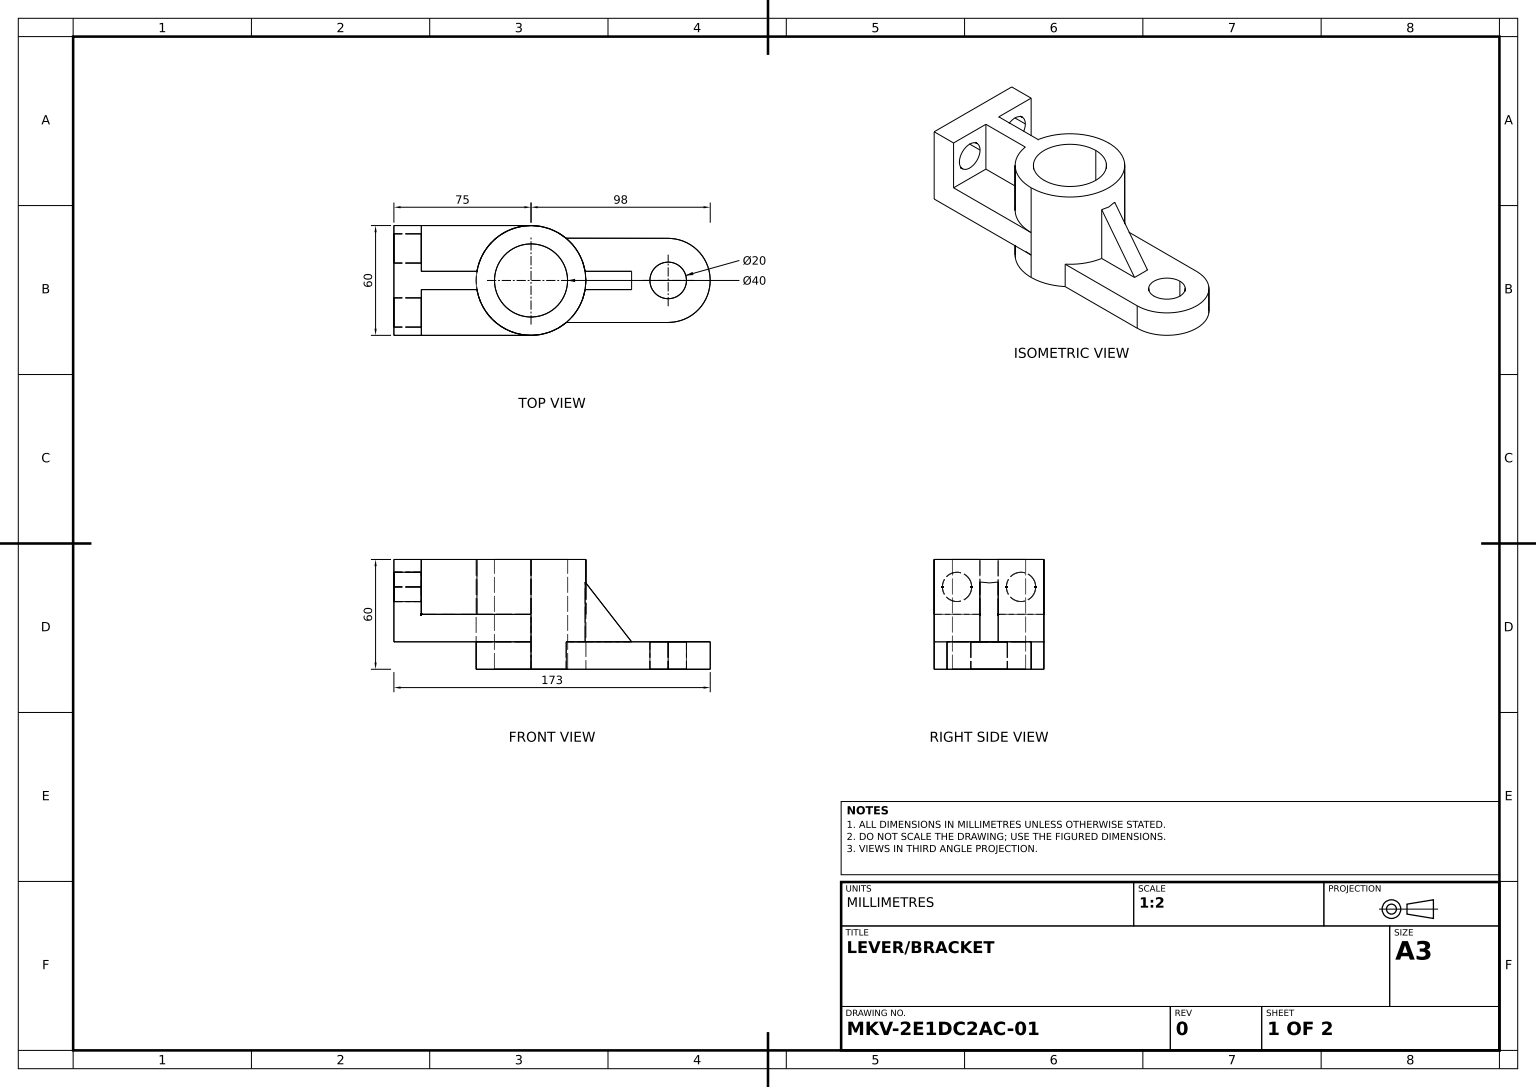
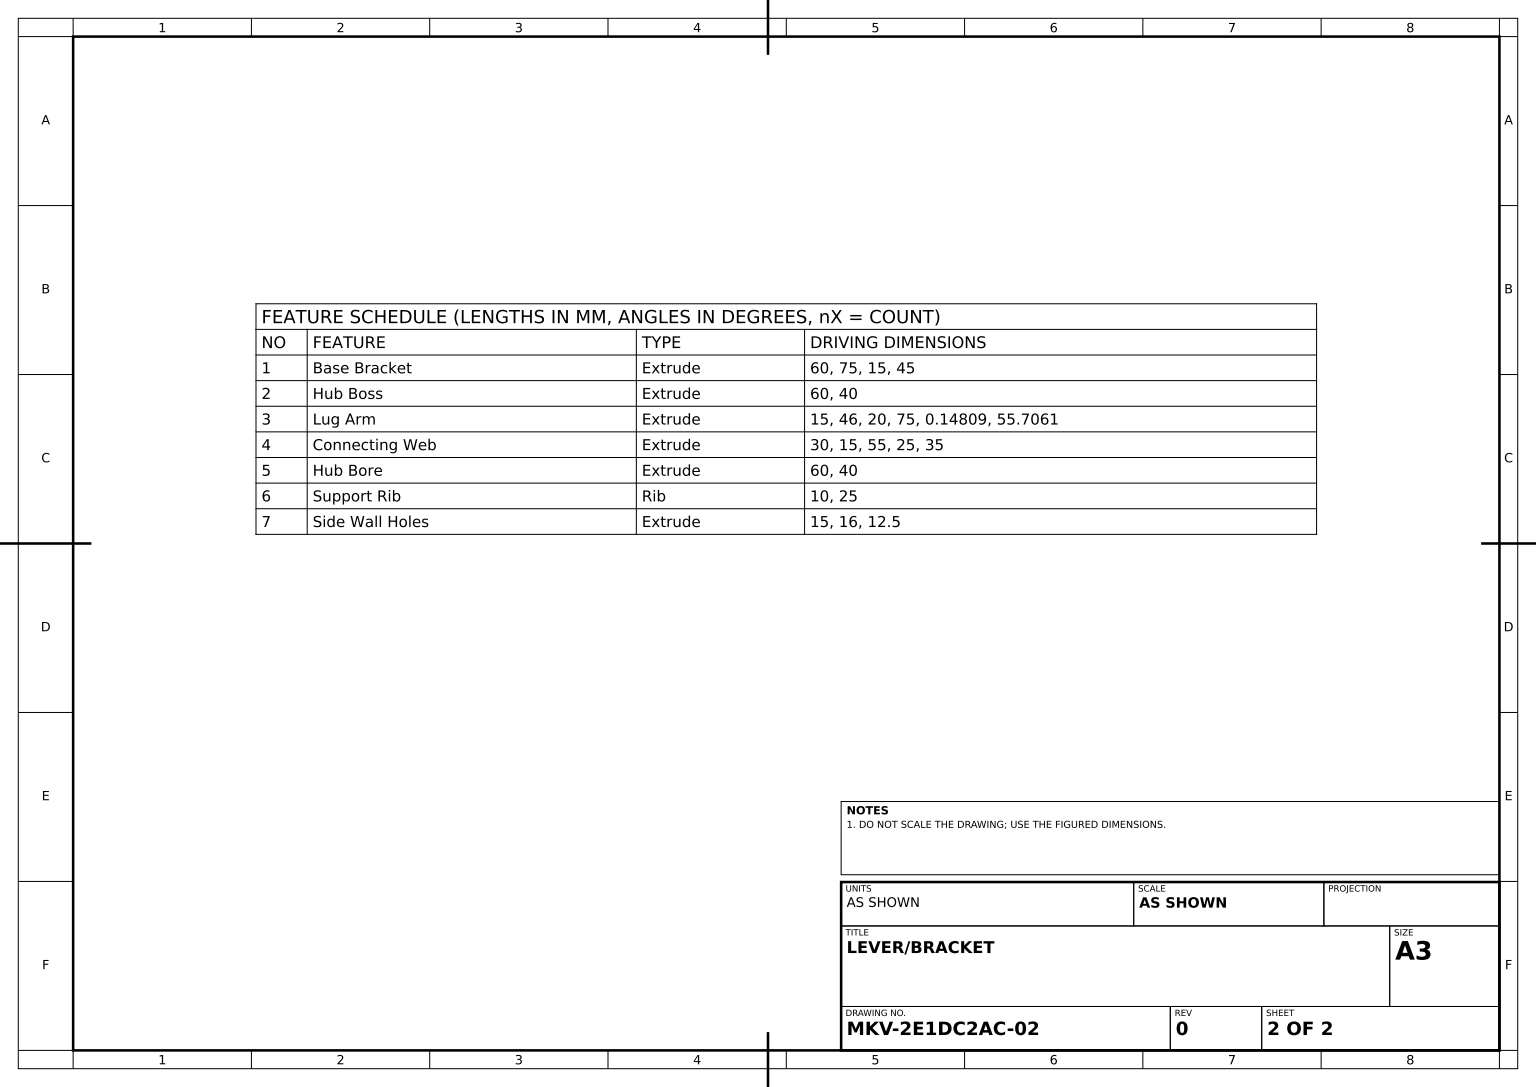
from build123d import *
from build123d.topology import SkipClean

# Parameters (mm, degrees)
BASE_BRACKET_DEPTH        = 30
HUB_BOSS_SKETCH_R         = 30
HUB_BOSS_SKETCH_R_2       = 20
HUB_BOSS_DEPTH            = 60
LUG_ARM_SKETCH_R          = 10
LUG_ARM_DEPTH             = 15
CONNECTING_WEB_SKETCH_W   = 40
CONNECTING_WEB_SKETCH_H   = 10
CONNECTING_WEB_DEPTH      = 30
HUB_START                 = -60
HUB_BORE_SKETCH_R         = 20
HUB_BORE_DEPTH            = 60
SUPPORT_RIB_REACH         = 120.76
SUPPORT_RIB_SKETCH_WALL_W = 296.52928849
SUPPORT_RIB_SKETCH_WALL_H = 10
SIDE_WALL_HOLES_SKETCH_R  = 8
SIDE_WALL_HOLES_DEPTH     = 15


with BuildPart() as part:
    # Base Bracket Profile Sketch → Base Bracket (new, symmetric)
    with BuildSketch(Plane.XY):
        Polygon((0, 15), (-75, 15), (-75, 60), (-60, 60), (-60, 30), (0, 30), align=None)
    extrude(amount=BASE_BRACKET_DEPTH, both=True)

    # Hub Boss Sketch → Hub Boss (add)
    with BuildSketch(Plane(origin=(0, 0, 0), x_dir=(1, 0, 0), z_dir=(0, 1, 0))):
        with Locations(Location((0, 0, 0), (0, 0, 270))):
            Circle(HUB_BOSS_SKETCH_R)
        with Locations(Location((0, 0, 0), (0, 0, 270))):
            Circle(HUB_BOSS_SKETCH_R_2, mode=Mode.SUBTRACT)
    extrude(amount=HUB_BOSS_DEPTH)

    # Lug Arm Sketch → Lug Arm (add)
    with BuildSketch(Plane(origin=(0, 0, 0), x_dir=(1, 0, 0), z_dir=(0, 1, 0))):
        with BuildLine():
            Line((74.999995036, 23.027288115), (19.14580869, 23.096276964))
            Line((19.14580869, 23.096276964), (19.293898223, 5.267398918))
            ThreePointArc((19.293898223, 5.267398918), (20, 0), (19.293898223, -5.267398918))
            Line((19.293898223, -5.267398918), (19.293898223, -22.972711885))
            Line((19.293898223, -22.972711885), (74.999995036, -22.972711885))
            ThreePointArc((74.999995036, -22.972711885), (97.999995036, 0.027288115), (74.999995036, 23.027288115))
        make_face()
        with Locations(Location((74.999995036, 0.027288115, 0), (0, 0, 270))):
            Circle(LUG_ARM_SKETCH_R, mode=Mode.SUBTRACT)
    extrude(amount=LUG_ARM_DEPTH)

    # Connecting Web Sketch → Connecting Web (add)
    with BuildSketch(Plane(origin=(0, 60, 0), x_dir=(1, 0, 0), z_dir=(0, 1, 0))):
        with Locations((-40, 0)):
            Rectangle(CONNECTING_WEB_SKETCH_W, CONNECTING_WEB_SKETCH_H)
    extrude(amount=-CONNECTING_WEB_DEPTH)

    # Hub Bore Sketch → Hub Bore (cut)
    with SkipClean():  # the faces are left unmerged after this step: merging them gives an invalid solid
        with BuildSketch(Plane(origin=(0, 60, 0), x_dir=(1, 0, 0), z_dir=(0, 1, 0)).offset(HUB_START)):
            with Locations(Location((0, 0, 0), (0, 0, 270))):
                Circle(HUB_BORE_SKETCH_R)
        extrude(amount=HUB_BORE_DEPTH, mode=Mode.SUBTRACT)

    # Support Rib Sketch wall → Support Rib (add, up to next)
    with BuildSketch(Plane(origin=(37.5, 37.5, 0), x_dir=(0.613940613515, -0.789352217376, 0), z_dir=(0.789352217376, 0.613940613515, 0)), mode=Mode.PRIVATE) as support_rib_sk1:
        Rectangle(SUPPORT_RIB_SKETCH_WALL_W, SUPPORT_RIB_SKETCH_WALL_H)
    support_rib_tool1 = extrude(support_rib_sk1.sketch, amount=-SUPPORT_RIB_REACH, mode=Mode.PRIVATE) - part.part
    add(support_rib_tool1.solids().sort_by_distance((37.5, 37.5, 0))[0])

    # Side Wall Holes Sketch → Side Wall Holes (cut)
    with SkipClean():  # the faces are left unmerged after this step: merging them gives an invalid solid
        with BuildSketch(Plane.ZY.offset(75)):
            with Locations((-17.5, 45)):
                Circle(SIDE_WALL_HOLES_SKETCH_R)
            with Locations((17.5, 45)):
                Circle(SIDE_WALL_HOLES_SKETCH_R)
        extrude(amount=-SIDE_WALL_HOLES_DEPTH, mode=Mode.SUBTRACT)


solid = part.part
